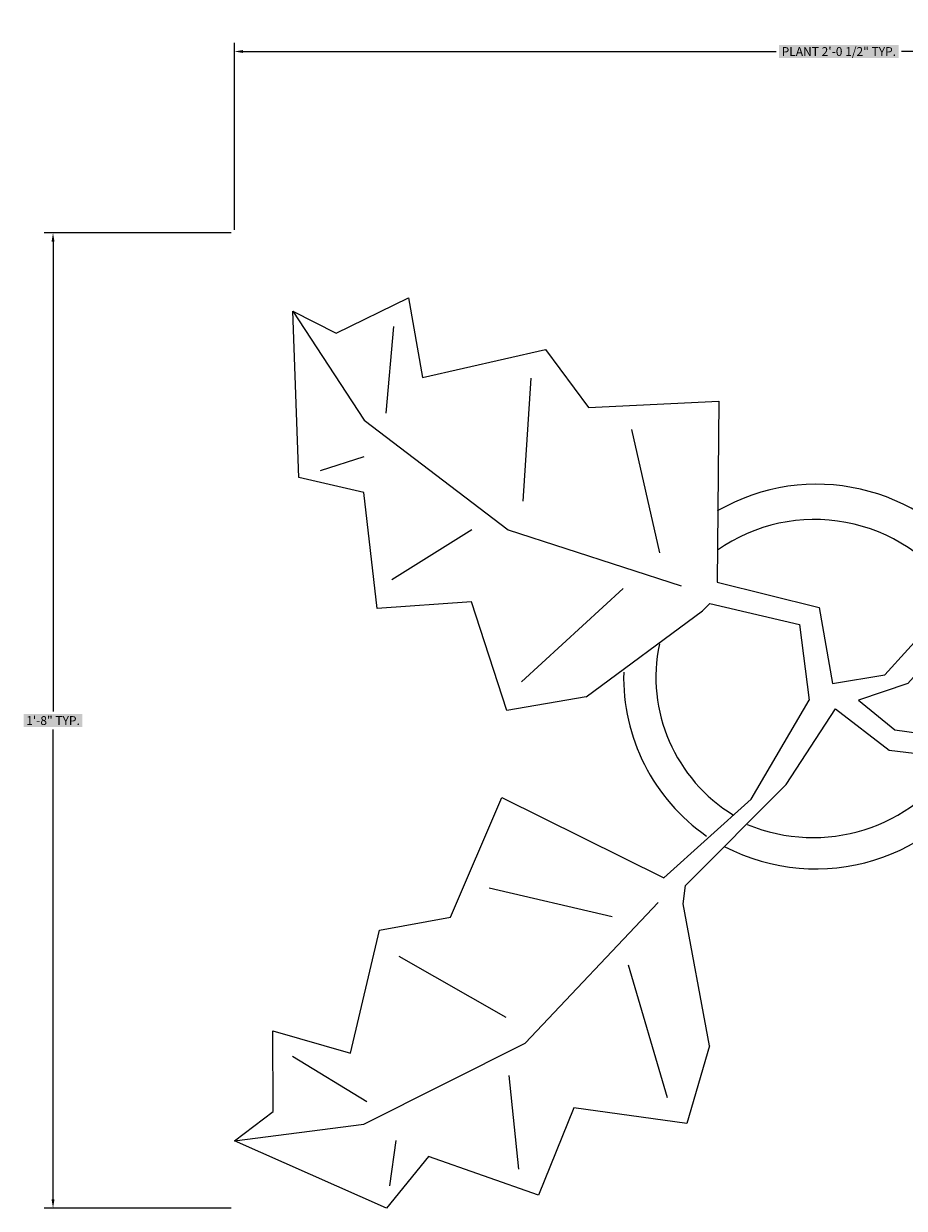
# Model space of a CAD drawing. Units: inches. Extents: x -301 to 715, y -607 to 364.
# Tile 88 of 141: x 97 to 115, y -255 to -231. Entities that reach past the tile are written whole.
import ezdxf

# ---------------------------------------------------------------- set-up
doc = ezdxf.new("R2010")
doc.units = ezdxf.units.IN
doc.header["$MEASUREMENT"] = 0
doc.layers.add('A-ANNO-DIMS', color=2, linetype='Continuous', lineweight=18)
doc.layers.add('L-PLNT', color=94, linetype='Continuous', lineweight=13)
doc.styles.get("Standard").update_dxf_attribs({"font": 'arial.ttf'})
doc.dimstyles.get("Standard").update_dxf_attribs({"dimtxt": 0.18, "dimasz": 0.18, "dimexe": 0.18, "dimexo": 0.0625, "dimgap": 0.09, "dimtad": 0, "dimtih": 1, "dimtoh": 1, "dimdec": 1, "dimzin": 0, "dimdsep": 46, "dimlunit": 4, "dimtxsty": 'Standard', "dimcen": 0.09, "dimclrd": 3, "dimclre": 4, "dimclrt": 6, "dimadec": 0, "dimazin": 0, "dimtfac": 1, "dimtdec": 1, "dimtofl": 0, "dimtmove": 0, "dimatfit": 3, "dimfxl": 1, "dimtfill": 2, "dimtfillclr": 51, "dimtolj": 1, "dimtzin": 0, "dimarcsym": 0})

# ---------------------------------------------------------------- blocks, each defined once
blk = doc.blocks.new('Plant - Rubber or Philodendron')
for p, q in [((13.3837, 12.301), (14.68, 13.9039)), ((14.68, 13.9039), (19.3848, 11.8146)), ((8.8871, 10.7908), (9.9809, 13.4933)), ((9.9809, 13.4933), (13.3837, 12.301)), ((14.5816, 13.2037), (14.3848, 11.8033)), ((10.5828, 12.6946), (10.8893, 9.7953)), ((-14.8639, 10.7964), (-12.6195, 11.8975)), ((-12.6195, 11.8975), (-12.1909, 9.4345)), ((19.3848, 11.8146), (15.3859, 11.3055)), ((19.3848, 11.8146), (18.1868, 10.9119)), ((-16.2005, 11.4774), (-13.9899, 8.1064)), ((-16.2005, 11.4774), (-14.8639, 10.7964)), ((-16.0159, 6.3329), (-16.2005, 11.4774)), ((-13.3174, 8.325), (-13.0735, 11.0065)), ((4.6914, 8.8812), (5.3859, 11.2828)), ((5.3859, 11.2828), (8.8871, 10.7908)), ((15.3859, 11.3055), (10.3916, 8.7942)), ((18.1868, 10.9119), (18.1925, 8.4119)), ((-12.1909, 9.4345), (-8.3829, 10.3)), ((-8.3829, 10.3), (-7.0549, 8.501)), ((5.9878, 10.4842), (7.1971, 6.3869)), ((15.2875, 10.6053), (17.5907, 9.2105)), ((-8.8369, 9.409), (-9.0894, 5.6095)), ((4.6914, 8.8812), (5.5014, 4.4831)), ((10.3916, 8.7942), (6.2847, 4.4028)), ((15.7909, 9.1065), (14.8995, 5.3044)), ((18.1925, 8.4119), (15.7909, 9.1065)), ((-7.0549, 8.501), (-3.0284, 8.6941)), ((-3.0284, 8.6941), (-3.0709, 3.1041)), ((-13.9899, 8.1064), (-9.5434, 4.7185)), ((-4.8529, 4.012), (-5.7184, 7.82)), ((14.2977, 6.1031), (10.9934, 7.9956)), ((-15.3434, 6.5514), (-13.9984, 6.9884)), ((-14.0069, 5.8704), (-16.0159, 6.3329)), ((-13.5868, 2.2894), (-14.0069, 5.8704)), ((14.8995, 5.3044), (12.7005, 4.8994)), ((7.7005, 4.8881), (11.5025, 3.9967)), ((12.7005, 4.8994), (11.1089, 1.1958)), ((-13.1329, 3.1804), (-10.6614, 4.727)), ((-9.5434, 4.7185), (-4.1917, 2.9888)), ((5.4346, 3.9146), (5.5014, 4.4831)), ((2.1141, 0.2298), (5.4346, 3.9146)), ((6.1032, 3.6844), (2.8262, -0.031)), ((11.1089, 1.1958), (6.1032, 3.6844)), ((-3.0709, 3.1041), (0.0797, 2.3163)), ((-9.1318, 0.0195), (-5.9793, 2.9025)), ((-10.6784, 2.491), (-13.5868, 2.2894)), ((-9.5858, -0.8715), (-10.6784, 2.491)), ((-7.1228, -0.443), (-3.5248, 2.2131)), ((-3.5248, 2.2131), (-3.3011, 2.4355)), ((-3.3011, 2.4355), (-0.5306, 1.7947)), ((0.0797, 2.3163), (0.4866, -0.031)), ((-0.5306, 1.7947), (-0.2255, -0.5527)), ((-0.5306, 1.7947), (-0.5306, 1.7947)), ((0.4866, -0.031), (2.1141, 0.2298)), ((2.8262, -0.031), (1.3003, -0.5527)), ((-7.1228, -0.443), (-9.5858, -0.8715)), ((-2.019, -3.6148), (-0.2255, -0.5527)), ((1.3003, -0.5527), (2.4193, -1.4655)), ((11.6605, -0.5413), (6.895, -2.1175)), ((11.6605, -0.5413), (14.1354, -0.8948)), ((-0.9375, -3.1608), (0.5883, -0.8135)), ((0.5883, -0.8135), (2.2447, -2.0916)), ((14.1354, -0.8948), (14.1354, -4.4304)), ((2.4193, -1.4655), (6.895, -2.1175)), ((2.2447, -2.0916), (6.7108, -2.6626)), ((8.3544, -2.7453), (13.1973, -2.1704)), ((4.943, -7.9659), (6.7108, -2.6626)), ((12.3677, -6.1981), (7.219, -2.6772)), ((-4.0579, -6.2781), (-0.9375, -3.1608)), ((-11.3237, -7.2629), (-9.7321, -3.5593)), ((-9.7321, -3.5593), (-4.7264, -6.0479)), ((-2.019, -3.6148), (-4.7264, -6.0479)), ((8.125, -4.0768), (7.7715, -7.9659)), ((14.1354, -4.4304), (16.9638, -5.1375)), ((16.9638, -5.1375), (16.2567, -8.673)), ((16.2567, -5.8446), (13.4283, -6.5517)), ((15.5496, -10.7943), (12.3677, -6.1981)), ((-6.3237, -7.2516), (-10.1257, -6.3602)), ((-4.1246, -6.8466), (-4.0579, -6.2781)), ((-9.0148, -11.1577), (-4.9047, -6.8122)), ((-3.3146, -11.2447), (-4.1246, -6.8466)), ((10.2463, -10.4408), (11.6605, -6.9053)), ((-13.5228, -7.6679), (-11.3237, -7.2629)), ((-14.4141, -11.4699), (-13.5228, -7.6679)), ((8.8321, -9.0266), (4.943, -7.9659)), ((-12.921, -8.4665), (-9.6166, -10.359)), ((-4.611, -12.8477), (-5.8203, -8.7504)), ((16.2567, -8.673), (18.0245, -9.7337)), ((9.5392, -11.1479), (8.8321, -9.0266)), ((17.3174, -9.7337), (15.9032, -9.7337)), ((18.0245, -9.7337), (16.6103, -14.6834)), ((-16.8157, -10.7754), (-14.4141, -11.4699)), ((-16.8101, -13.2754), (-16.8157, -10.7754)), ((14.8425, -10.7943), (13.7819, -13.2692)), ((16.6103, -14.6834), (15.5496, -10.7943)), ((-14.0091, -13.669), (-9.0148, -11.1577)), ((-3.3146, -11.2447), (-4.0092, -13.6463)), ((13.4283, -11.5015), (9.5392, -11.1479)), ((-13.9107, -12.9688), (-16.2139, -11.574)), ((13.0748, -13.9763), (13.4283, -11.5015)), ((-9.206, -15.0581), (-9.5126, -12.1588)), ((-7.5103, -13.1543), (-8.6042, -15.8568)), ((-4.0092, -13.6463), (-7.5103, -13.1543)), ((-18.008, -14.1781), (-16.8101, -13.2754)), ((-18.008, -14.1781), (-14.0091, -13.669)), ((15.5496, -13.6228), (13.0748, -13.9763)), ((16.6103, -14.6834), (15.5496, -13.6228)), ((-13.3032, -16.2674), (-18.008, -14.1781)), ((-13.2048, -15.5672), (-13.008, -14.1668)), ((-12.0069, -14.6645), (-13.3032, -16.2674)), ((-8.6042, -15.8568), (-12.0069, -14.6645))]:
    blk.add_line(p, q)
for centre, radius, start, end in [((0, 0), 6.1275, 34.37569, 120.1028), ((-0.0601, -0.2075), 5.2461, 33.82192, 124.9414), ((-0.098, 0.1364), 6.1288, 341.2017, 26.09184), ((-0.2664, 0.1682), 5.2775, 338.4094, 20.03007), ((0.0308, 0.1664), 5, 168.1647, 238.6725), ((0.0308, 0.1664), 6, 178.6147, 235.1169), ((-0.1102, 0.4886), 5.2883, 247.3711, 327.472), ((-0.0234, 0.3825), 6.1492, 242.5812, 331.2714)]:
    blk.add_arc(centre, radius, start, end)
blk = doc.blocks.new('*D106')
at = {"layer": 'A-ANNO-DIMS', "color": 4, "lineweight": -2, "transparency": 16777216}
for p, q in [((101.18, -235.449), (101.18, -231.622)), ((125.91, -235.449), (125.91, -231.622))]:
    blk.add_line(p, q, dxfattribs=at)
at = {"layer": 'A-ANNO-DIMS', "color": 3, "lineweight": -2, "transparency": 16777216}
for p, q in [((101.36, -231.802), (112.261, -231.802)), ((125.73, -231.802), (114.829, -231.802))]:
    blk.add_line(p, q, dxfattribs=at)
at = {"layer": 'A-ANNO-DIMS', "color": 3, "transparency": 16777216}
for points in [[(101.36, -231.772), (101.36, -231.832), (101.18, -231.802)], [(125.73, -231.772), (125.73, -231.832), (125.91, -231.802)]]:
    blk.add_solid(points, dxfattribs=at)
at = {"layer": 'Defpoints', "color": 0, "transparency": 16777216}
for p in [(125.91, -231.802), (101.18, -235.511), (125.91, -235.511)]:
    blk.add_point(p, dxfattribs=at)
at = {"layer": 'A-ANNO-DIMS', "color": 6, "transparency": 16777216, "insert": (113.545, -231.802), "char_height": 0.18, "attachment_point": 5, "bg_fill": 1, "box_fill_scale": 1.25, "bg_fill_color": 51, "bg_fill_transparency": 0}
blk.add_mtext('\\A1;PLANT 2\'-0 1/2" TYP.', dxfattribs=at)
blk = doc.blocks.new('*D107')
at = {"layer": 'A-ANNO-DIMS', "color": 4, "lineweight": -2, "transparency": 16777216}
for p, q in [((101.118, -235.511), (97.291, -235.511)), ((101.118, -255.465), (97.291, -255.465))]:
    blk.add_line(p, q, dxfattribs=at)
at = {"layer": 'A-ANNO-DIMS', "color": 3, "lineweight": -2, "transparency": 16777216}
for p, q in [((97.471, -235.691), (97.471, -245.306)), ((97.471, -255.285), (97.471, -245.67))]:
    blk.add_line(p, q, dxfattribs=at)
at = {"layer": 'A-ANNO-DIMS', "color": 3, "transparency": 16777216}
for points in [[(97.441, -235.691), (97.501, -235.691), (97.471, -235.511)], [(97.441, -255.285), (97.501, -255.285), (97.471, -255.465)]]:
    blk.add_solid(points, dxfattribs=at)
at = {"layer": 'Defpoints', "color": 0, "transparency": 16777216}
for p in [(97.471, -235.511), (101.18, -235.511), (101.18, -255.465)]:
    blk.add_point(p, dxfattribs=at)
at = {"layer": 'A-ANNO-DIMS', "color": 6, "transparency": 16777216, "insert": (97.471, -245.488), "char_height": 0.18, "attachment_point": 5, "bg_fill": 1, "box_fill_scale": 1.25, "bg_fill_color": 51, "bg_fill_transparency": 0}
blk.add_mtext('\\A1;1\'-8" TYP.', dxfattribs=at)

msp = doc.modelspace()

# ---------------------------------------------------------------- block references
at = {"layer": 'L-PLNT', "xscale": 0.6613521884636907, "yscale": 0.6613521884636907, "zscale": 0.6613521884636907}
msp.add_blockref('Plant - Rubber or Philodendron', (113.09, -244.707), dxfattribs=at)

# ---------------------------------------------------------------- dimensions: what is measured, and where the dimension line sits
at = {"layer": 'A-ANNO-DIMS'}
dim = msp.add_linear_dim(base=(125.91, -231.802), p1=(101.18, -235.511), p2=(125.91, -235.511), text='PLANT <> TYP.', dimstyle='Standard', override={"dimdec": 1, "dimlfac": 1, "dimrnd": 0, "dimzin": 1, "dimdsep": 46, "dimlunit": 4, "dimfrac": 2}, dxfattribs=at)
dim.commit()
dim.dimension.update_dxf_attribs({"geometry": '*D106', "text_midpoint": (113.545, -231.802)})
dim = msp.add_linear_dim(base=(97.471, -235.511), p1=(101.18, -255.465), p2=(101.18, -235.511), angle=90, text='<> TYP.', dimstyle='Standard', override={"dimdec": 1, "dimlfac": 1, "dimrnd": 0, "dimzin": 1, "dimdsep": 46, "dimlunit": 4, "dimfrac": 2}, dxfattribs=at)
dim.commit()
dim.dimension.update_dxf_attribs({"geometry": '*D107', "text_midpoint": (97.471, -245.488)})

doc.saveas('drawing.dxf')
